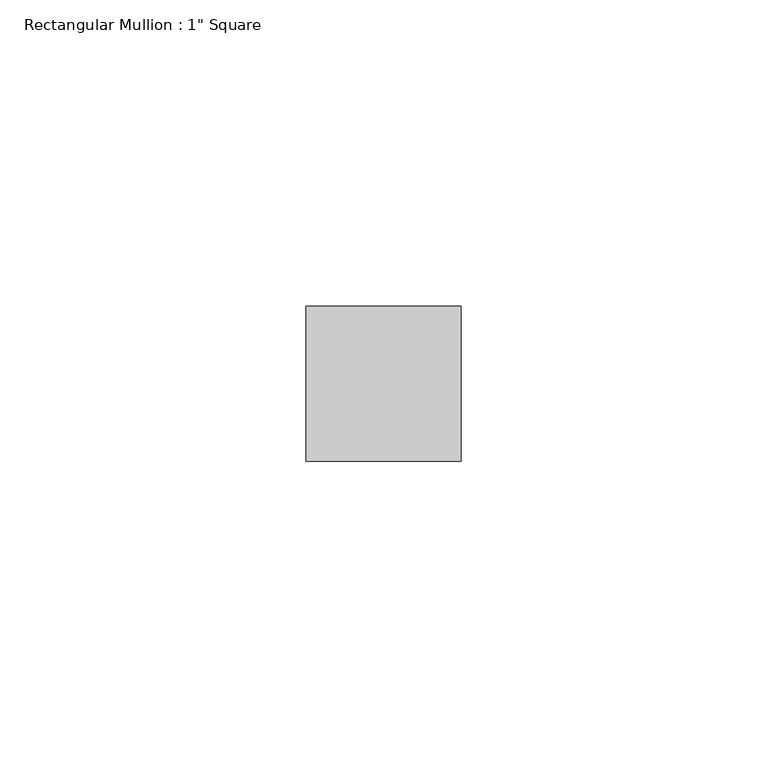
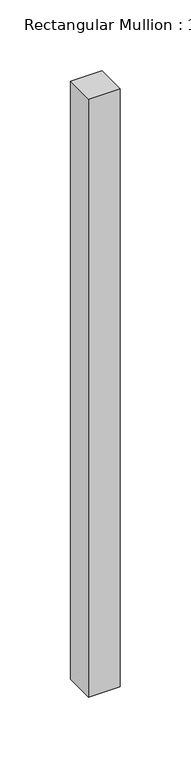
"""IFC4 building model written with IfcOpenShell, lengths in millimetres: member geometry."""

from ifc_helpers import new_model, si_unit, frame, origin, place, context, project, spatial, polyline, outline, extrude, source, transform, mapped, element, save


def member_9625144b(model_context):
    return source(origin(), model_context, "Body", "SweptSolid", [
        extrude(outline(polyline([(12.7, 12.7), (12.7, -12.7), (-12.7, -12.7), (-12.7, 12.7), (12.7, 12.7)])), frame((0.0, 0.0, -514.35), z_axis=(0.0, 0.0, 1.0), x_axis=(1.0, 0.0, 0.0)), (0.0, 0.0, 1.0), 514.35),
    ])


if __name__ == "__main__":
    model = new_model("IFC4")
    model_context = context("Model", 3, world=origin())
    ifc_project = project(units=[si_unit("LENGTHUNIT", "METRE", prefix="MILLI")], contexts=[model_context])
    site = spatial("IfcSite", under=ifc_project)
    building = spatial("IfcBuilding", under=site)
    placement = place(None, origin())
    member_shape = member_9625144b(model_context)
    element("IfcMember", 1, ObjectType="Rectangular Mullion : 1\" Square", at=placement, inside=building, context=model_context, shape_type="MappedRepresentation", body=[
        mapped(member_shape, transform((0.0, 0.0, 0.0), x_axis=(1.0, 0.0, 0.0), y_axis=(0.0, 1.0, 0.0), z_axis=(0.0, 0.0, 1.0))),
    ])
    save(model, "model.ifc")

# Revit data of these elements
# Type "Rectangular Mullion : 1\" Square"
#   built-in parameter 1007304 = 0.0833333 (stored number, unit not read)
#   built-in parameter 1007301 = 0.0416667 (stored number, unit not read)
#   built-in parameter 1007300 = 0.0416667 (stored number, unit not read)
